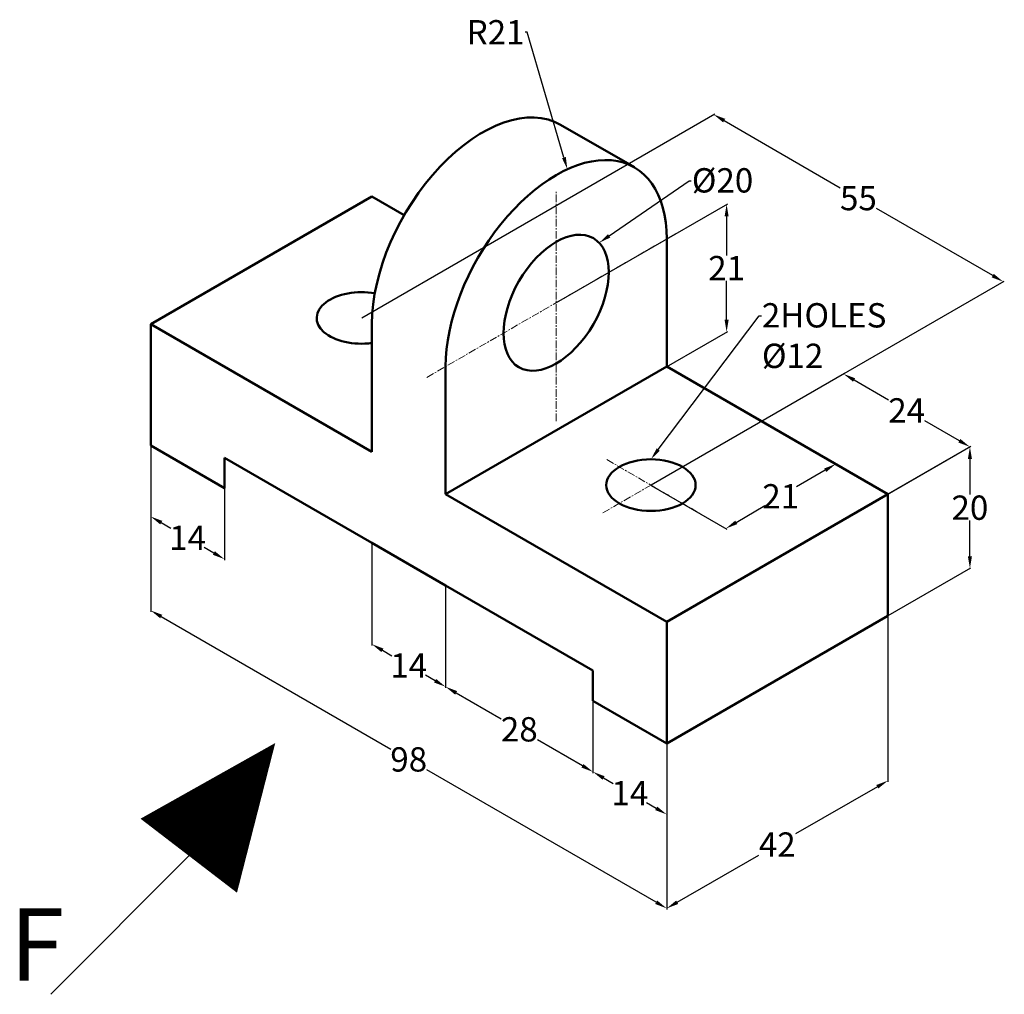
# Model space of a CAD drawing. Units: millimetres. Extents: x -145 to 168, y -286 to 127.
# Tile 2 of 2: x -81 to 81, y -33 to 127. Entities that reach past the tile are written whole.
import ezdxf
from ezdxf import colors
from ezdxf.entities.mleader import LeaderData, LeaderLine
from ezdxf.math import Vec2, Vec3

# ---------------------------------------------------------------- set-up
doc = ezdxf.new("R2010")
doc.units = ezdxf.units.MM
doc.header["$MEASUREMENT"] = 0
doc.linetypes.add('CENTER', pattern=[2, 1.25, -0.25, 0.25, -0.25])
for name, color, linetype, lineweight in [('M-CNTR', 1, 'CENTER', 18), ('M-DIMS', 2, 'Continuous', 25), ('M-OUTL', 7, 'Continuous', 50), ('M-TEXT', 3, 'Continuous', 25)]:
    doc.layers.add(name, color=color, linetype=linetype, lineweight=lineweight)
doc.styles.get("Standard").update_dxf_attribs({"font": 'arial.ttf'})
doc.dimstyles.get("Standard").update_dxf_attribs({"dimtxt": 4, "dimasz": 2, "dimexe": 0.18, "dimexo": 0.0625, "dimgap": 0.09, "dimtad": 0, "dimtih": 1, "dimtoh": 1, "dimdec": 0, "dimzin": 0, "dimdsep": 46, "dimtxsty": 'Standard', "dimcen": 0.09, "dimadec": 0, "dimazin": 0, "dimtfac": 1, "dimtdec": 0, "dimtofl": 0, "dimtmove": 0, "dimatfit": 3, "dimfxl": 1, "dimtolj": 1, "dimtzin": 0, "dimarcsym": 0})

# ---------------------------------------------------------------- blocks, each defined once
blk = doc.blocks.new('*D1')
at = {"layer": 'Defpoints', "color": 0, "transparency": 16777216}
for p in [(62.04, 29.33), (25.66, 8.33), (62.04, 2.21)]:
    blk.add_point(p, dxfattribs=at)
at = {"layer": 'M-DIMS', "color": 0, "lineweight": -2, "transparency": 16777216}
for p, q in [((62.04, 29.26), (62.04, 2.01)), ((25.66, 8.26), (25.66, -18.99)), ((60.31, 1.21), (46.87, -6.54)), ((27.4, -17.79), (40.84, -10.03))]:
    blk.add_line(p, q, dxfattribs=at)
at = {"layer": 'M-DIMS', "color": 0, "transparency": 16777216}
for points in [[(60.14, 1.5), (60.47, 0.93), (62.04, 2.21)], [(27.23, -17.5), (27.56, -18.07), (25.66, -18.79)]]:
    blk.add_solid(points, dxfattribs=at)
at = {"layer": 'M-DIMS', "color": 0, "transparency": 16777216, "insert": (43.85, -8.29), "char_height": 4, "attachment_point": 5}
blk.add_mtext('\\A1;42', dxfattribs=at)
blk = doc.blocks.new('*D2')
at = {"layer": 'Defpoints', "color": 0, "transparency": 16777216}
for p in [(75.53, 57.12), (62.04, 49.33), (62.04, 29.33)]:
    blk.add_point(p, dxfattribs=at)
at = {"layer": 'M-DIMS', "color": 0, "lineweight": -2, "transparency": 16777216}
for p, q in [((62.1, 49.37), (75.71, 57.23)), ((75.53, 55.12), (75.53, 49.26)), ((75.53, 39.12), (75.53, 44.99)), ((62.1, 29.37), (75.71, 37.23))]:
    blk.add_line(p, q, dxfattribs=at)
at = {"layer": 'M-DIMS', "color": 0, "transparency": 16777216}
for points in [[(75.2, 55.12), (75.87, 55.12), (75.53, 57.12)], [(75.2, 39.12), (75.87, 39.12), (75.53, 37.12)]]:
    blk.add_solid(points, dxfattribs=at)
at = {"layer": 'M-DIMS', "color": 0, "transparency": 16777216, "insert": (75.53, 47.12), "char_height": 4, "attachment_point": 5}
blk.add_mtext('\\A1;20', dxfattribs=at)
blk = doc.blocks.new('*D3')
at = {"layer": 'Defpoints', "color": 0, "transparency": 16777216}
for p in [(13.54, 15.33), (25.66, 8.33), (13.54, 3.66)]:
    blk.add_point(p, dxfattribs=at)
at = {"layer": 'M-DIMS', "color": 0, "lineweight": -2, "transparency": 16777216}
for p, q in [((13.54, 15.26), (13.54, 3.46)), ((25.66, 8.26), (25.66, -3.54)), ((15.27, 2.66), (16.84, 1.76)), ((23.93, -2.34), (22.36, -1.43))]:
    blk.add_line(p, q, dxfattribs=at)
at = {"layer": 'M-DIMS', "color": 0, "transparency": 16777216}
for points in [[(15.44, 2.95), (15.11, 2.37), (13.54, 3.66)], [(24.1, -2.05), (23.77, -2.63), (25.66, -3.34)]]:
    blk.add_solid(points, dxfattribs=at)
at = {"layer": 'M-DIMS', "color": 0, "transparency": 16777216, "insert": (19.6, 0.16), "char_height": 4, "attachment_point": 5}
blk.add_mtext('\\A1;14', dxfattribs=at)
blk = doc.blocks.new('*D4')
at = {"layer": 'Defpoints', "color": 0, "transparency": 16777216}
for p in [(-10.71, 34.33), (13.54, 20.33), (-10.71, 17.66)]:
    blk.add_point(p, dxfattribs=at)
at = {"layer": 'M-DIMS', "color": 0, "lineweight": -2, "transparency": 16777216}
for p, q in [((-10.71, 34.26), (-10.71, 17.46)), ((13.54, 20.26), (13.54, 3.46)), ((-8.98, 16.66), (-1.58, 12.39)), ((11.81, 4.66), (4.41, 8.94))]:
    blk.add_line(p, q, dxfattribs=at)
at = {"layer": 'M-DIMS', "color": 0, "transparency": 16777216}
for points in [[(-8.81, 16.95), (-9.14, 16.37), (-10.71, 17.66)], [(11.97, 4.95), (11.64, 4.37), (13.54, 3.66)]]:
    blk.add_solid(points, dxfattribs=at)
at = {"layer": 'M-DIMS', "color": 0, "transparency": 16777216, "insert": (1.42, 10.66), "char_height": 4, "attachment_point": 5}
blk.add_mtext('\\A1;28', dxfattribs=at)
blk = doc.blocks.new('*D5')
at = {"layer": 'Defpoints', "color": 0, "transparency": 16777216}
for p in [(-22.83, 41.33), (-10.71, 34.33), (-22.83, 24.66)]:
    blk.add_point(p, dxfattribs=at)
at = {"layer": 'M-DIMS', "color": 0, "lineweight": -2, "transparency": 16777216}
for p, q in [((-22.83, 41.26), (-22.83, 24.46)), ((-10.71, 34.26), (-10.71, 17.46)), ((-21.1, 23.66), (-19.53, 22.76)), ((-12.44, 18.66), (-14.01, 19.57))]:
    blk.add_line(p, q, dxfattribs=at)
at = {"layer": 'M-DIMS', "color": 0, "transparency": 16777216}
for points in [[(-20.93, 23.95), (-21.27, 23.37), (-22.83, 24.66)], [(-12.27, 18.95), (-12.61, 18.37), (-10.71, 17.66)]]:
    blk.add_solid(points, dxfattribs=at)
at = {"layer": 'M-DIMS', "color": 0, "transparency": 16777216, "insert": (-16.77, 21.16), "char_height": 4, "attachment_point": 5}
blk.add_mtext('\\A1;14', dxfattribs=at)
blk = doc.blocks.new('*D6')
at = {"layer": 'Defpoints', "color": 0, "transparency": 16777216}
for p in [(-59.21, 57.33), (-47.08, 50.33), (-59.21, 45.66)]:
    blk.add_point(p, dxfattribs=at)
at = {"layer": 'M-DIMS', "color": 0, "lineweight": -2, "transparency": 16777216}
for p, q in [((-59.21, 57.26), (-59.21, 45.46)), ((-47.08, 50.26), (-47.08, 38.46)), ((-57.47, 44.66), (-55.9, 43.76)), ((-48.81, 39.66), (-50.39, 40.57))]:
    blk.add_line(p, q, dxfattribs=at)
at = {"layer": 'M-DIMS', "color": 0, "transparency": 16777216}
for points in [[(-57.31, 44.95), (-57.64, 44.37), (-59.21, 45.66)], [(-48.65, 39.95), (-48.98, 39.37), (-47.08, 38.66)]]:
    blk.add_solid(points, dxfattribs=at)
at = {"layer": 'M-DIMS', "color": 0, "transparency": 16777216, "insert": (-53.14, 42.16), "char_height": 4, "attachment_point": 5}
blk.add_mtext('\\A1;14', dxfattribs=at)
blk = doc.blocks.new('*D7')
at = {"layer": 'Defpoints', "color": 0, "transparency": 16777216}
for p in [(75.53, 57.12), (23.07, 50.83), (43.85, 38.83)]:
    blk.add_point(p, dxfattribs=at)
at = {"layer": 'M-DIMS', "color": 0, "lineweight": -2, "transparency": 16777216}
for p, q in [((23.13, 50.87), (54.93, 69.23)), ((56.48, 68.12), (62.16, 64.85)), ((73.8, 58.12), (68.12, 61.4)), ((43.91, 38.87), (75.71, 57.23))]:
    blk.add_line(p, q, dxfattribs=at)
at = {"layer": 'M-DIMS', "color": 0, "transparency": 16777216}
for points in [[(56.65, 68.41), (56.31, 67.84), (54.75, 69.12)], [(73.97, 58.41), (73.63, 57.84), (75.53, 57.12)]]:
    blk.add_solid(points, dxfattribs=at)
at = {"layer": 'M-DIMS', "color": 0, "transparency": 16777216, "insert": (65.14, 63.12), "char_height": 4, "attachment_point": 5}
blk.add_mtext('\\A1;24', dxfattribs=at)
blk = doc.blocks.new('*D8')
at = {"layer": 'Defpoints', "color": 0, "transparency": 16777216}
for p in [(41.11, 61.42), (53.45, 54.29), (23.04, 50.82)]:
    blk.add_point(p, dxfattribs=at)
at = {"layer": 'M-DIMS', "color": 0, "lineweight": -2, "transparency": 16777216}
for p, q in [((41.17, 61.38), (53.63, 54.19)), ((51.73, 53.28), (47.02, 50.52)), ((23.1, 50.78), (35.56, 43.59)), ((37.11, 44.7), (41.82, 47.46))]:
    blk.add_line(p, q, dxfattribs=at)
at = {"layer": 'M-DIMS', "color": 0, "transparency": 16777216}
for points in [[(51.56, 53.56), (51.9, 52.99), (53.45, 54.29)], [(36.94, 44.99), (37.28, 44.42), (35.39, 43.69)]]:
    blk.add_solid(points, dxfattribs=at)
at = {"layer": 'M-DIMS', "color": 0, "transparency": 16777216, "insert": (44.42, 48.99), "char_height": 4, "attachment_point": 5}
blk.add_mtext('\\A1;21', dxfattribs=at)
blk = doc.blocks.new('*D9')
at = {"layer": 'Defpoints', "color": 0, "transparency": 16777216}
for p in [(7.48, 80.83), (35.52, 76.02), (7.48, 59.83)]:
    blk.add_point(p, dxfattribs=at)
at = {"layer": 'M-DIMS', "color": 0, "lineweight": -2, "transparency": 16777216}
for p, q in [((7.54, 80.87), (35.7, 97.12)), ((35.52, 95.02), (35.52, 88.62)), ((35.52, 78.02), (35.52, 84.42)), ((7.54, 59.87), (35.7, 76.12))]:
    blk.add_line(p, q, dxfattribs=at)
at = {"layer": 'M-DIMS', "color": 0, "transparency": 16777216}
for points in [[(35.18, 95.02), (35.85, 95.02), (35.52, 97.02)], [(35.18, 78.02), (35.85, 78.02), (35.52, 76.02)]]:
    blk.add_solid(points, dxfattribs=at)
at = {"layer": 'M-DIMS', "color": 0, "transparency": 16777216, "insert": (35.52, 86.52), "char_height": 4, "attachment_point": 5}
blk.add_mtext('\\A1;21', dxfattribs=at)
blk = doc.blocks.new('*D10')
at = {"layer": 'Defpoints', "color": 0, "transparency": 16777216}
for p in [(81.01, 84.29), (-24.56, 78.33), (23.07, 50.83)]:
    blk.add_point(p, dxfattribs=at)
at = {"layer": 'M-DIMS', "color": 0, "lineweight": -2, "transparency": 16777216}
for p, q in [((-24.5, 78.37), (33.56, 111.89)), ((35.11, 110.79), (54.22, 99.75)), ((79.28, 85.29), (60.16, 96.32)), ((23.13, 50.87), (81.19, 84.39))]:
    blk.add_line(p, q, dxfattribs=at)
at = {"layer": 'M-DIMS', "color": 0, "transparency": 16777216}
for points in [[(35.28, 111.08), (34.94, 110.5), (33.38, 111.79)], [(79.45, 85.58), (79.11, 85), (81.01, 84.29)]]:
    blk.add_solid(points, dxfattribs=at)
at = {"layer": 'M-DIMS', "color": 0, "transparency": 16777216, "insert": (57.19, 98.04), "char_height": 4, "attachment_point": 5}
blk.add_mtext('\\A1;55', dxfattribs=at)
blk = doc.blocks.new('*D11')
at = {"layer": 'Defpoints', "color": 0, "transparency": 16777216}
for p in [(-59.21, 57.33), (-59.21, 30.21), (25.66, 8.33)]:
    blk.add_point(p, dxfattribs=at)
at = {"layer": 'M-DIMS', "color": 0, "lineweight": -2, "transparency": 16777216}
for p, q in [((-59.21, 57.26), (-59.21, 30.01)), ((-57.47, 29.21), (-19.73, 7.42)), ((25.66, 8.26), (25.66, -18.99)), ((23.93, -17.79), (-13.81, 4.01))]:
    blk.add_line(p, q, dxfattribs=at)
at = {"layer": 'M-DIMS', "color": 0, "transparency": 16777216}
for points in [[(-57.31, 29.5), (-57.64, 28.93), (-59.21, 30.21)], [(24.1, -17.5), (23.77, -18.07), (25.66, -18.79)]]:
    blk.add_solid(points, dxfattribs=at)
at = {"layer": 'M-DIMS', "color": 0, "transparency": 16777216, "insert": (-16.77, 5.71), "char_height": 4, "attachment_point": 5}
blk.add_mtext('\\A1;98', dxfattribs=at)

msp = doc.modelspace()

# ---------------------------------------------------------------- linework, layer by layer
at = {"layer": 'M-CNTR'}
for p, q in [((7.48, 61.37), (7.48, 99.05)), ((-13.79, 68.55), (27.32, 92.29)), ((15.16, 46.27), (30.92, 55.37)), ((15.81, 55.02), (31, 46.25))]:
    msp.add_line(p, q, dxfattribs=at)
at = {"layer": 'M-OUTL'}
for p, q in [((8.21, 110.11), (20.34, 103.11)), ((-59.21, 77.33), (-22.83, 98.33)), ((-22.83, 98.33), (-17.51, 95.26)), ((25.66, 70.33), (25.66, 91.33)), ((-59.21, 57.33), (-59.21, 77.33)), ((-59.21, 77.33), (-22.83, 56.33)), ((-22.83, 56.33), (-22.83, 77.33)), ((25.66, 70.33), (-10.71, 49.33)), ((-10.71, 49.33), (-10.71, 70.33)), ((62.04, 49.33), (25.66, 70.33)), ((-47.08, 50.33), (-59.21, 57.33)), ((-22.83, 41.33), (-47.08, 55.33)), ((-47.08, 55.33), (-47.08, 50.33)), ((25.66, 28.33), (-10.71, 49.33)), ((62.04, 49.33), (25.66, 28.33)), ((62.04, 29.33), (62.04, 49.33)), ((-10.71, 34.33), (-22.83, 41.33)), ((13.54, 20.33), (-10.71, 34.33)), ((25.66, 8.33), (62.04, 29.33)), ((25.66, 28.33), (25.66, 8.33)), ((13.54, 15.33), (13.54, 20.33)), ((25.66, 8.33), (13.54, 15.33))]:
    msp.add_line(p, q, dxfattribs=at)
for centre, major_axis, start_param, end_param in [((-4.65, 87.83), (-12.86, -22.27), 3.141593, 5.497787), ((7.48, 80.83), (-12.86, -22.27), 2.356194, 5.497787), ((-24.56, 78.33), (-7.35, 0), 4.407229, 8.091923)]:
    msp.add_ellipse(centre, major_axis=major_axis, ratio=0.57735, start_param=start_param, end_param=end_param, dxfattribs=at)
for centre, major_axis in [((7.48, 80.83), (-6.12, -10.61)), ((23.07, 50.83), (-7.35, 0))]:
    msp.add_ellipse(centre, major_axis=major_axis, ratio=0.57735, dxfattribs=at)
at = {"layer": 'M-TEXT'}
msp.add_lwpolyline([(-52.95, -10.13, 20, 0, 0), (-38.72, 8.41, 0, 0, 0)], format="xyseb", dxfattribs=at)
msp.add_lwpolyline([(-52.95, -10.13), (-75.61, -32.93)], dxfattribs=at)

# ---------------------------------------------------------------- texts
msp.add_text('F', height=11.87, dxfattribs=at).set_placement((-82.39, -30.68))

# ---------------------------------------------------------------- dimensions: what is measured, and where the dimension line sits
at = {"layer": 'M-DIMS'}
for p1, p2, distance, picture, middle in [((-24.56, 78.33), (23.07, 50.83), 57.94, '*D10', (57.19, 98.04)), ((7.48, 80.83), (7.48, 59.83), 28.04, '*D9', (35.52, 86.52)), ((23.07, 50.83), (43.85, 38.83), 31.68, '*D7', (65.14, 63.12)), ((23.04, 50.82), (41.11, 61.42), -12.39, '*D8', (44.42, 48.99)), ((-47.08, 50.33), (-59.21, 57.33), 10.11, '*D6', (-53.14, 42.16)), ((25.66, 8.33), (-59.21, 57.33), 23.49, '*D11', (-16.77, 5.71)), ((62.04, 29.33), (62.04, 49.33), -13.5, '*D2', (75.53, 47.12)), ((-10.71, 34.33), (-22.83, 41.33), 14.44, '*D5', (-16.77, 21.16)), ((13.54, 20.33), (-10.71, 34.33), 14.44, '*D4', (1.42, 10.66)), ((25.66, 8.33), (62.04, 29.33), -23.49, '*D1', (43.85, -8.29)), ((25.66, 8.33), (13.54, 15.33), 10.11, '*D3', (19.6, 0.16))]:
    dim = msp.add_aligned_dim(p1=p1, p2=p2, distance=distance, dimstyle='Standard', override={"dimclrd": 0, "dimclre": 0, "dimclrt": 0}, dxfattribs=at)
    dim.commit()
    dim.dimension.update_dxf_attribs({"geometry": picture, "text_midpoint": middle})

# ---------------------------------------------------------------- leaders
at = {"layer": 'M-TEXT'}
ml = msp.add_multileader_mtext('Standard', dxfattribs=at)
ml.set_content('R21', color=256)
ml.set_leader_properties()
ml.build(insert=Vec2(0, 0))
ml.multileader.update_dxf_attribs({"dogleg_length": 0.36, "arrow_head_size": 2})
ctx = ml.context
ctx.base_point, ctx.arrow_head_size, ctx.landing_gap_size, ctx.plane_origin = Vec3(-6.6, 125.32), 2, 0.09, Vec3(9.32, 102.79)
ctx.text_align_type = 2
notes = []
notes.append((ctx, [(0, (1, 1, 0), (2.73, 125.32), (-1, 0), 0.36, [(0, [(9.32, 102.79)], 0, [])])]))
ctx.mtext.insert, ctx.mtext.alignment, ctx.mtext.flow_direction = Vec3(2.28, 127.32), 3, 5
ml = msp.add_multileader_mtext('Standard', dxfattribs=at)
ml.set_content('%%C20', color=256)
ml.set_leader_properties()
ml.build(insert=Vec2(0, 0))
ml.multileader.update_dxf_attribs({"dogleg_length": 0.36, "arrow_head_size": 2})
ctx = ml.context
ctx.base_point, ctx.arrow_head_size, ctx.landing_gap_size, ctx.plane_origin = Vec3(29.7, 100.88), 2, 0.09, Vec3(14.55, 90.69)
notes.append((ctx, [(0, (1, 1, 0), (29.34, 100.88), (1, 0), 0.36, [(0, [(14.55, 90.69)], 0, [])])]))
ctx.mtext.insert, ctx.mtext.flow_direction = Vec3(29.79, 102.96), 5
ml = msp.add_multileader_mtext('Standard', dxfattribs=at)
ml.set_content('2HOLES\\P%%C12', color=256)
ml.set_leader_properties()
ml.build(insert=Vec2(0, 0))
ml.multileader.update_dxf_attribs({"dogleg_length": 0.36, "arrow_head_size": 2})
ctx = ml.context
ctx.base_point, ctx.arrow_head_size, ctx.landing_gap_size, ctx.plane_origin = Vec3(41.23, 78.68), 2, 0.09, Vec3(23.07, 55.08)
notes.append((ctx, [(0, (1, 1, 0), (40.87, 78.68), (1, 0), 0.36, [(0, [(23.07, 55.08)], 0, [])])]))
ctx.mtext.insert, ctx.mtext.flow_direction = Vec3(41.32, 80.76), 5
for ctx, leaders in notes:
    for number, flags, end, landing, length, lines in leaders:
        leader = LeaderData()
        leader.index, (leader.has_last_leader_line, leader.has_dogleg_vector, leader.attachment_direction) = number, flags
        leader.last_leader_point, leader.dogleg_vector, leader.dogleg_length = Vec3(end), Vec3(landing), length
        for number, points, colour, breaks in lines:
            line = LeaderLine()
            line.index, line.vertices, line.color, line.breaks = number, Vec3.list(points), colors.encode_raw_color(colour), breaks
            leader.lines.append(line)
        ctx.leaders.append(leader)

doc.saveas('drawing.dxf')
